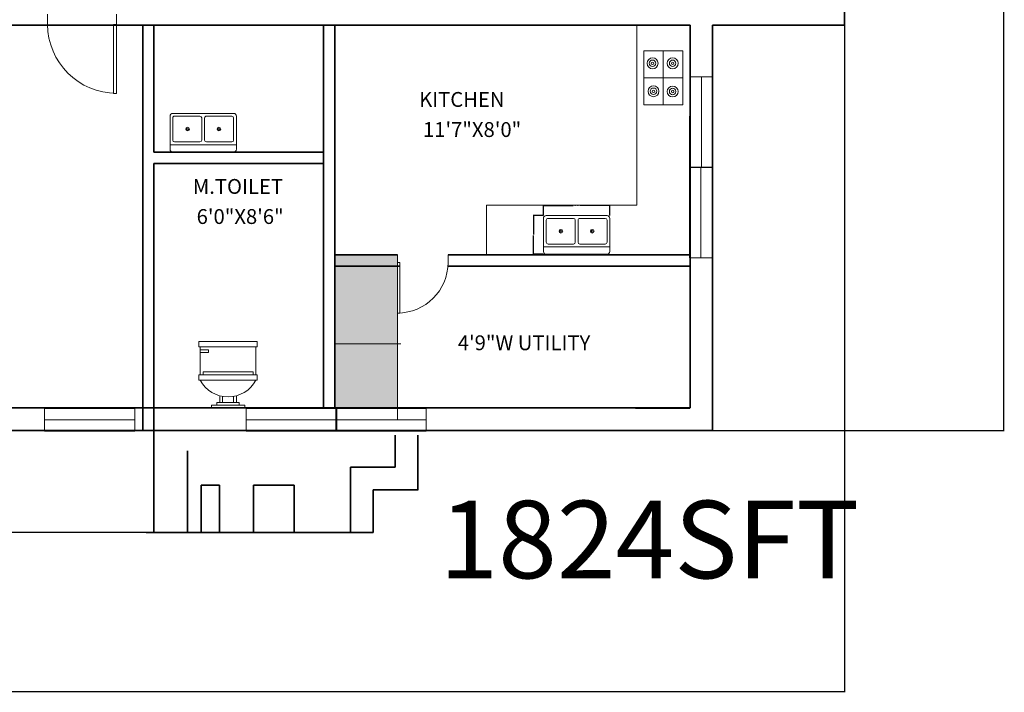
# Model space of a CAD drawing. Units: millimetres. Extents: x 27017497 to 27018854, y 7058029 to 7059154.
# Tile 89 of 91: x 27018462 to 27018854, y 7058029 to 7058297. Entities that reach past the tile are written whole.
import ezdxf

# ---------------------------------------------------------------- set-up
doc = ezdxf.new("R2010")
doc.units = ezdxf.units.MM
for name, color, linetype, lineweight in [('A-ANNO-DIMS', 2, 'Continuous', 18), ('A-AREA-IDEN', 7, 'Continuous', 18), ('A-DOOR', 4, 'Continuous', 20), ('A-EQPM', 9, 'Continuous', 18), ('A-FLOR-CASE', 8, 'Continuous', 20), ('A-FLOR-CASE-PATT', 44, 'Continuous', 13), ('A-FLOR-FIXT', 9, 'Continuous', 18), ('A-GLAZ', 4, 'Continuous', 18), ('A-WALL', 7, 'Continuous', 35)]:
    doc.layers.add(name, color=color, linetype=linetype, lineweight=lineweight)
doc.styles.get("Standard").update_dxf_attribs({"font": 'arial.ttf'})
doc.dimstyles.get("Standard").update_dxf_attribs({"dimtxt": 0.18, "dimasz": 0.18, "dimexe": 0.18, "dimexo": 0.0625, "dimgap": 0.09, "dimtad": 0, "dimtih": 1, "dimtoh": 1, "dimdec": 4, "dimzin": 0, "dimdsep": 46, "dimtxsty": 'Standard', "dimcen": 0.09, "dimadec": 0, "dimazin": 0, "dimtfac": 1, "dimtdec": 4, "dimtofl": 0, "dimtmove": 0, "dimatfit": 3, "dimfxl": 1, "dimtolj": 1, "dimtzin": 0, "dimarcsym": 0})

# ---------------------------------------------------------------- blocks, each defined once
blk = doc.blocks.new('*U2')
for p, q in [((0, 0), (0, -6)), ((40, 0), (40, -6))]:
    blk.add_line(p, q)
blk.add_lwpolyline([(0, 0), (0, 40), (1.75, 40), (1.75, 0)], close=True)
blk.add_arc((0, 0), 40, 0, 90)
blk = doc.blocks.new('*U6')
for p, q in [((-10, 22), (-10, 12)), ((10, 12), (10, 22)), ((-10, 21), (-7, 21)), ((-7, 20), (-10, 20)), ((-7, 21), (-7, 20)), ((10.5, 12), (-10.5, 12)), ((-10.5, 10), (-10.5, 12)), ((9, 13), (-9, 13)), ((-9, 13), (-9, 12)), ((9, 12), (9, 13)), ((10.5, 12), (10.5, 10)), ((10.5, 10), (-10.5, 10)), ((-3, 4.4065), (-3, 2)), ((-2, 2), (-2, 4.1658)), ((2, 4.1658), (2, 2)), ((3, 2), (3, 4.4065)), ((4, 2), (-4, 2)), ((-4, 2), (-4, 1)), ((4, 1), (4, 2))]:
    blk.add_line(p, q)
for points in [[(10.5, 22), (10.5, 24), (-10.5, 24), (-10.5, 22)], [(6, 0), (6, 1), (-6, 1), (-6, 0)]]:
    blk.add_lwpolyline(points, close=True)
blk.add_arc((0, 15.3333), 11.3333, 208.0725, 331.9275)
blk = doc.blocks.new('Sink-double - 36 in top')
for p, q in [((-18, -4), (18, -4)), ((-0.75, -18.5), (-0.75, -6.5)), ((0.75, -6.5), (0.75, -18.5))]:
    blk.add_line(p, q)
for points in [[(-16.5, 0), (16.5, 0)], [(-18, -19.5), (-18, -1.5)], [(18, -1.5), (18, -19.5)], [(-16.5, -18.5), (-16.5, -6.5)], [(-15.5, -5.5), (-1.75, -5.5)], [(1.75, -5.5), (15.5, -5.5)], [(16.5, -6.5), (16.5, -18.5)], [(16.5, -21), (-16.5, -21)], [(-1.75, -19.5), (-15.5, -19.5)], [(15.5, -19.5), (1.75, -19.5)]]:
    blk.add_lwpolyline(points)
for centre, radius in [((-8.5, -12.5), 1), ((-8.5, -12.5), 0.5), ((8.5, -12.5), 1), ((8.5, -12.5), 0.5)]:
    blk.add_circle(centre, radius)
for centre, radius, start, end in [((-16.5, -1.5), 1.5, 90, 180), ((16.5, -1.5), 1.5, 0, 90), ((-15.5, -6.5), 1, 90, 180), ((-1.75, -6.5), 1, 0, 90), ((1.75, -6.5), 1, 90, 180), ((15.5, -6.5), 1, 0, 90), ((-16.5, -19.5), 1.5, 180, 270), ((-15.5, -18.5), 1, 180, 270), ((-1.75, -18.5), 1, 270, 0), ((1.75, -18.5), 1, 180, 270), ((15.5, -18.5), 1, 270, 0), ((16.5, -19.5), 1.5, 270, 0)]:
    blk.add_arc(centre, radius, start, end)
blk = doc.blocks.new('COOKTOP-FOUR-BURNER')
for points in [[(7.75, 21.43), (7.75, 10.72), (0, 10.72), (0, 21.43)], [(15.51, 21.43), (15.51, 10.72), (7.75, 10.72), (7.75, 21.43)], [(7.75, 10.72), (7.75, 0), (0, 0), (0, 10.72)], [(15.51, 10.72), (15.51, 0), (7.75, 0), (7.75, 10.72)]]:
    blk.add_lwpolyline(points, close=True)
for centre, radius in [((3.5, 16.51), 2.17), ((3.5, 16.51), 1.3), ((3.5, 16.51), 0.515), ((3.5, 16.51), 0.515), ((11.5, 16.51), 2.17), ((11.5, 16.51), 1.3), ((11.5, 16.51), 0.515), ((11.5, 16.51), 0.515), ((3.88, 5.36), 2.17), ((3.88, 5.36), 1.3), ((3.88, 5.36), 0.515), ((3.88, 5.36), 0.515), ((11.5, 5.27), 2.17), ((11.5, 5.27), 1.3), ((11.5, 5.27), 0.515), ((11.5, 5.27), 0.515)]:
    blk.add_circle(centre, radius)
blk = doc.blocks.new('WINDOW-SINGLE-LIGHT')
blk.add_lwpolyline([(36, 4.5), (36, 0), (0, 0), (0, 9), (36, 9), (36, 4.5), (0, 4.5)])
blk = doc.blocks.new('*D23')
at = {"layer": 'A-ANNO-DIMS', "color": 0, "lineweight": -2, "transparency": 16777216}
for p, q in [((27018670.72, 7058218.66), (27018670.72, 7058222.74)), ((27018670.9, 7058222.56), (27018682.52, 7058222.56)), ((27018696.96, 7058222.56), (27018685.33, 7058222.56)), ((27018697.14, 7058218.66), (27018697.14, 7058222.74))]:
    blk.add_line(p, q, dxfattribs=at)
at = {"layer": 'A-ANNO-DIMS', "color": 0, "transparency": 16777216}
for points in [[(27018670.9, 7058222.59), (27018670.9, 7058222.53), (27018670.72, 7058222.56)], [(27018696.96, 7058222.59), (27018696.96, 7058222.53), (27018697.14, 7058222.56)]]:
    blk.add_solid(points, dxfattribs=at)
at = {"layer": 'Defpoints', "color": 0, "transparency": 16777216}
for p in [(27018670.72, 7058222.56), (27018670.72, 7058218.59), (27018697.14, 7058218.59)]:
    blk.add_point(p, dxfattribs=at)
at = {"layer": 'A-ANNO-DIMS', "color": 0, "transparency": 16777216, "insert": (27018683.93, 7058222.56), "char_height": 0.18, "attachment_point": 5}
blk.add_mtext('\\A1;DOUBLE SINK 26 TYP.', dxfattribs=at)
blk = doc.blocks.new('*D24')
at = {"layer": 'A-ANNO-DIMS', "color": 0, "lineweight": -2, "transparency": 16777216}
for p, q in [((27018670.65, 7058218.59), (27018666.57, 7058218.59)), ((27018666.75, 7058218.41), (27018666.75, 7058211.07)), ((27018666.75, 7058203.36), (27018666.75, 7058210.71)), ((27018670.65, 7058203.18), (27018666.57, 7058203.18))]:
    blk.add_line(p, q, dxfattribs=at)
at = {"layer": 'A-ANNO-DIMS', "color": 0, "transparency": 16777216}
for points in [[(27018666.72, 7058218.41), (27018666.78, 7058218.41), (27018666.75, 7058218.59)], [(27018666.72, 7058203.36), (27018666.78, 7058203.36), (27018666.75, 7058203.18)]]:
    blk.add_solid(points, dxfattribs=at)
at = {"layer": 'Defpoints', "color": 0, "transparency": 16777216}
for p in [(27018670.72, 7058218.59), (27018666.75, 7058203.18), (27018670.72, 7058203.18)]:
    blk.add_point(p, dxfattribs=at)
at = {"layer": 'A-ANNO-DIMS', "color": 0, "transparency": 16777216, "insert": (27018666.75, 7058210.89), "char_height": 0.18, "attachment_point": 5}
blk.add_mtext('\\A1;15 TYP.', dxfattribs=at)
blk = doc.blocks.new('*D47')
at = {"layer": 'A-ANNO-DIMS', "color": 0, "lineweight": -2, "transparency": 16777216}
for p, q in [((27017561.17, 7058294.35), (27017561.17, 7058028.6)), ((27018790.61, 7058294.35), (27018790.61, 7058028.6)), ((27017561.35, 7058028.78), (27018175.43, 7058028.78)), ((27018790.43, 7058028.78), (27018176.34, 7058028.78))]:
    blk.add_line(p, q, dxfattribs=at)
at = {"layer": 'A-ANNO-DIMS', "color": 0, "transparency": 16777216}
for points in [[(27017561.35, 7058028.81), (27017561.35, 7058028.75), (27017561.17, 7058028.78)], [(27018790.43, 7058028.81), (27018790.43, 7058028.75), (27018790.61, 7058028.78)]]:
    blk.add_solid(points, dxfattribs=at)
at = {"layer": 'Defpoints', "color": 0, "transparency": 16777216}
for p in [(27017561.17, 7058294.41), (27018790.61, 7058294.41), (27018790.61, 7058028.78)]:
    blk.add_point(p, dxfattribs=at)
at = {"layer": 'A-ANNO-DIMS', "color": 0, "transparency": 16777216, "insert": (27018175.89, 7058028.78), "char_height": 0.18, "attachment_point": 5}
blk.add_mtext('\\A1;1229.4', dxfattribs=at)
blk = doc.blocks.new('*D48')
at = {"layer": 'A-ANNO-DIMS', "color": 0, "lineweight": -2, "transparency": 16777216}
for p, q in [((27018463.5, 7058622.91), (27017497.54, 7058622.91)), ((27017497.72, 7058622.73), (27017497.72, 7058357.75)), ((27017497.72, 7058092.41), (27017497.72, 7058357.39)), ((27018555.13, 7058092.23), (27017497.54, 7058092.23))]:
    blk.add_line(p, q, dxfattribs=at)
at = {"layer": 'A-ANNO-DIMS', "color": 0, "transparency": 16777216}
for points in [[(27017497.69, 7058622.73), (27017497.75, 7058622.73), (27017497.72, 7058622.91)], [(27017497.69, 7058092.41), (27017497.75, 7058092.41), (27017497.72, 7058092.23)]]:
    blk.add_solid(points, dxfattribs=at)
at = {"layer": 'Defpoints', "color": 0, "transparency": 16777216}
for p in [(27018463.56, 7058622.91), (27017497.72, 7058092.23), (27018555.19, 7058092.23)]:
    blk.add_point(p, dxfattribs=at)
at = {"layer": 'A-ANNO-DIMS', "color": 0, "transparency": 16777216, "insert": (27017497.72, 7058357.57), "char_height": 0.18, "attachment_point": 5}
blk.add_mtext('\\A1;530.7', dxfattribs=at)
blk = doc.blocks.new('*D53')
at = {"layer": 'A-ANNO-DIMS', "color": 0, "lineweight": -2, "transparency": 16777216}
for p, q in [((27018738.17, 7058589.91), (27018854.24, 7058589.91)), ((27018854.06, 7058589.73), (27018854.06, 7058361.59)), ((27018854.06, 7058133.09), (27018854.06, 7058361.23)), ((27018738.17, 7058132.91), (27018854.24, 7058132.91))]:
    blk.add_line(p, q, dxfattribs=at)
at = {"layer": 'A-ANNO-DIMS', "color": 0, "transparency": 16777216}
for points in [[(27018854.03, 7058589.73), (27018854.09, 7058589.73), (27018854.06, 7058589.91)], [(27018854.03, 7058133.09), (27018854.09, 7058133.09), (27018854.06, 7058132.91)]]:
    blk.add_solid(points, dxfattribs=at)
at = {"layer": 'Defpoints', "color": 0, "transparency": 16777216}
for p in [(27018738.11, 7058589.91), (27018854.06, 7058589.91), (27018738.11, 7058132.91)]:
    blk.add_point(p, dxfattribs=at)
at = {"layer": 'A-ANNO-DIMS', "color": 0, "transparency": 16777216, "insert": (27018854.06, 7058361.41), "char_height": 0.18, "attachment_point": 5}
blk.add_mtext('\\A1;457', dxfattribs=at)

msp = doc.modelspace()

# ---------------------------------------------------------------- hatches: boundary and pattern name
at = {"layer": 'A-FLOR-CASE-PATT'}
h = msp.add_hatch(color=256, dxfattribs=at)
h.dxf.hatch_style = 1
h.paths.add_polyline_path([(27018612.584, 7058198.412), (27018587.606, 7058198.412), (27018587.606, 7058167.535), (27018612.584, 7058167.535)])
h.paths.add_polyline_path([(27018612.584, 7058167.535), (27018587.606, 7058167.535), (27018587.606, 7058141.912), (27018612.584, 7058141.912)])
h.paths.add_polyline_path([(27018612.584, 7058202.912), (27018587.606, 7058202.912), (27018587.606, 7058198.412), (27018612.584, 7058198.412), (27018612.584, 7058199.894)])

# ---------------------------------------------------------------- linework, layer by layer
at = {"layer": 'A-FLOR-CASE'}
for p, q in [((27018707.848, 7058294.412), (27018707.848, 7058222.72)), ((27018707.848, 7058222.72), (27018648.02, 7058222.72)), ((27018648.02, 7058222.72), (27018648.02, 7058202.912)), ((27018612.584, 7058198.342), (27018612.584, 7058137.344)), ((27018587.606, 7058167.535), (27018613.96, 7058167.535))]:
    msp.add_line(p, q, dxfattribs=at)
at = {"layer": 'A-WALL'}
for p, q in [((27018790.606, 7058437.098), (27018790.606, 7058294.412)), ((27018549.606, 7058294.412), (27018319.606, 7058294.412)), ((27018511.106, 7058294.412), (27018511.106, 7058132.912)), ((27018515.606, 7058294.412), (27018515.606, 7058243.912)), ((27018592.99, 7058294.412), (27018549.606, 7058294.412)), ((27018583.106, 7058294.412), (27018583.106, 7058141.912)), ((27018587.606, 7058294.412), (27018587.606, 7058141.912)), ((27018729.106, 7058294.412), (27018593.007, 7058294.412)), ((27018729.106, 7058294.412), (27018729.106, 7058141.912)), ((27018738.106, 7058294.412), (27018738.106, 7058132.912)), ((27018790.606, 7058294.412), (27018738.106, 7058294.412)), ((27018729.08, 7058258.237), (27018729.08, 7058207.055)), ((27018583.106, 7058243.912), (27018515.606, 7058243.912)), ((27018583.106, 7058239.412), (27018515.606, 7058239.412)), ((27018515.606, 7058239.412), (27018515.606, 7058092.317)), ((27018612.584, 7058202.912), (27018587.606, 7058202.912)), ((27018729.106, 7058202.912), (27018632.711, 7058202.912)), ((27018613.465, 7058198.412), (27018587.606, 7058198.412)), ((27018729.106, 7058198.412), (27018632.656, 7058198.412)), ((27018468.106, 7058141.912), (27018319.606, 7058141.912)), ((27018549.606, 7058141.912), (27018468.106, 7058141.912)), ((27018729.106, 7058141.912), (27018549.606, 7058141.912)), ((27018729.048, 7058141.888), (27018707.31, 7058141.888)), ((27018468.106, 7058132.912), (27018310.606, 7058132.912)), ((27018545.106, 7058132.912), (27018468.106, 7058132.912)), ((27018549.606, 7058132.912), (27018468.106, 7058132.912)), ((27018738.106, 7058132.912), (27018549.606, 7058132.912)), ((27018738.106, 7058132.912), (27018549.606, 7058132.912)), ((27018729.048, 7058132.888), (27018707.31, 7058132.888)), ((27018611.669, 7058131.088), (27018611.669, 7058118.346)), ((27018620.669, 7058131.088), (27018620.669, 7058121.039)), ((27018528.894, 7058092.317), (27018528.894, 7058124.857)), ((27018620.67, 7058121.044), (27018620.67, 7058109.226)), ((27018593.921, 7058118.346), (27018593.921, 7058092.317)), ((27018593.921, 7058118.346), (27018611.669, 7058118.346)), ((27018541.65, 7058111.139), (27018534.342, 7058111.139)), ((27018571.47, 7058111.139), (27018555.192, 7058111.139)), ((27018602.921, 7058109.346), (27018602.921, 7058092.317)), ((27018602.921, 7058109.346), (27018620.67, 7058109.346)), ((27018602.921, 7058092.317), (27018512.505, 7058092.317))]:
    msp.add_line(p, q, dxfattribs=at)
for points in [[(27018541.65, 7058111.139), (27018541.65, 7058092.317), (27018534.342, 7058092.317), (27018534.342, 7058111.139)], [(27018571.47, 7058111.139), (27018571.47, 7058092.23), (27018555.192, 7058092.23), (27018555.192, 7058111.139)]]:
    msp.add_lwpolyline(points, dxfattribs=at)

# ---------------------------------------------------------------- block references
at = {"layer": 'A-DOOR', "rotation": 180}
for p, xscale, yscale, zscale in [((27018500.714, 7058294.79), 0.6870473523349573, 0.6870473523349573, 0.6870473523349573), ((27018612.584, 7058199.894), -0.503175151877956, 0.503175151877956, 0.503175151877956)]:
    msp.add_blockref('*U2', p, dxfattribs=dict(at, xscale=xscale, yscale=yscale, zscale=zscale))
at = {"layer": 'A-EQPM'}
msp.add_blockref('COOKTOP-FOUR-BURNER', (27018710.671, 7058262.762), dxfattribs=at)
at = {"layer": 'A-FLOR-FIXT', "xscale": 0.7340308267416257, "yscale": 0.7340308267416257, "zscale": 0.7340308267416257, "rotation": 180}
for p in [(27018535.206, 7058243.912), (27018683.928, 7058203.18)]:
    msp.add_blockref('Sink-double - 36 in top', p, dxfattribs=at)
at = {"layer": 'A-FLOR-FIXT', "xscale": 1.105119395603938, "yscale": 1.105119395603938, "zscale": 1.105119395603938}
msp.add_blockref('*U6', (27018545.106, 7058141.912), dxfattribs=at)
at = {"layer": 'A-GLAZ', "extrusion": (0, 0, -1), "zscale": -1, "rotation": 270}
for p in [(-27018738.125, 7058273.913), (-27018737.906, 7058237.7)]:
    msp.add_blockref('WINDOW-SINGLE-LIGHT', p, dxfattribs=at)
at = {"layer": 'A-GLAZ', "extrusion": (0, 0, -1), "zscale": -1}
for p in [(-27018507.972, 7058132.679), (-27018588.361, 7058132.679), (-27018624.048, 7058132.679)]:
    msp.add_blockref('WINDOW-SINGLE-LIGHT', p, dxfattribs=at)

# ---------------------------------------------------------------- texts
at = {"layer": 'A-ANNO-DIMS'}
for s, p in [('11\'7"X8\'0"', (27018622.735, 7058249.917)), ('6\'0"X8\'6"', (27018532.597, 7058215.254))]:
    msp.add_text(s, height=5.9118, dxfattribs=at).set_placement(p)
at = {"layer": 'A-AREA-IDEN'}
for s, height, p in [('KITCHEN', 5.9118, (27018621.2, 7058261.914)), ('M.TOILET', 5.9118, (27018531.062, 7058227.251)), ('4\'9"W UTILITY', 5.91176, (27018636.597, 7058164.937)), ('1824SFT', 30.9043, (27018629.259, 7058074.038))]:
    msp.add_text(s, height=height, dxfattribs=at).set_placement(p)

# ---------------------------------------------------------------- dimensions: what is measured, and where the dimension line sits
at = {"layer": 'A-ANNO-DIMS'}
for base, p1, p2, override, picture, middle in [((27017497.716, 7058092.23), (27018463.561, 7058622.912), (27018555.192, 7058092.23), {"dimdec": 1, "dimlfac": 1, "dimrnd": 0, "dimzin": 0, "dimdsep": 46, "dimlunit": 2}, '*D48', (27017497.716, 7058357.571)), ((27018854.056, 7058589.912), (27018738.106, 7058132.912), (27018738.106, 7058589.912), {"dimdec": 0, "dimlfac": 1, "dimrnd": 0, "dimzin": 0, "dimdsep": 46, "dimlunit": 2}, '*D53', (27018854.056, 7058361.412))]:
    dim = msp.add_linear_dim(base=base, p1=p1, p2=p2, angle=90, dimstyle='Standard', override=override, dxfattribs=at)
    dim.commit()
    dim.dimension.update_dxf_attribs({"geometry": picture, "text_midpoint": middle})
dim = msp.add_linear_dim(base=(27018790.606, 7058028.78), p1=(27017561.166, 7058294.412), p2=(27018790.606, 7058294.412), dimstyle='Standard', override={"dimdec": 1, "dimlfac": 1, "dimrnd": 0, "dimzin": 0, "dimdsep": 46, "dimlunit": 2}, dxfattribs=at)
dim.commit()
dim.dimension.update_dxf_attribs({"geometry": '*D47', "text_midpoint": (27018175.886, 7058028.78)})
for base, p1, p2, angle, text, picture, middle in [((27018670.715, 7058222.558), (27018697.141, 7058218.594), (27018670.715, 7058218.594), 180, 'DOUBLE SINK <> TYP.', '*D23', (27018683.928, 7058222.558)), ((27018666.752, 7058203.18), (27018670.715, 7058218.594), (27018670.715, 7058203.18), 270, '<> TYP.', '*D24', (27018666.752, 7058210.887))]:
    dim = msp.add_linear_dim(base=base, p1=p1, p2=p2, angle=angle, text=text, dimstyle='Standard', override={"dimdec": 0, "dimlfac": 1, "dimrnd": 0, "dimzin": 0, "dimdsep": 46, "dimlunit": 2}, dxfattribs=at)
    dim.commit()
    dim.dimension.update_dxf_attribs({"geometry": picture, "text_midpoint": middle})

doc.saveas('drawing.dxf')
